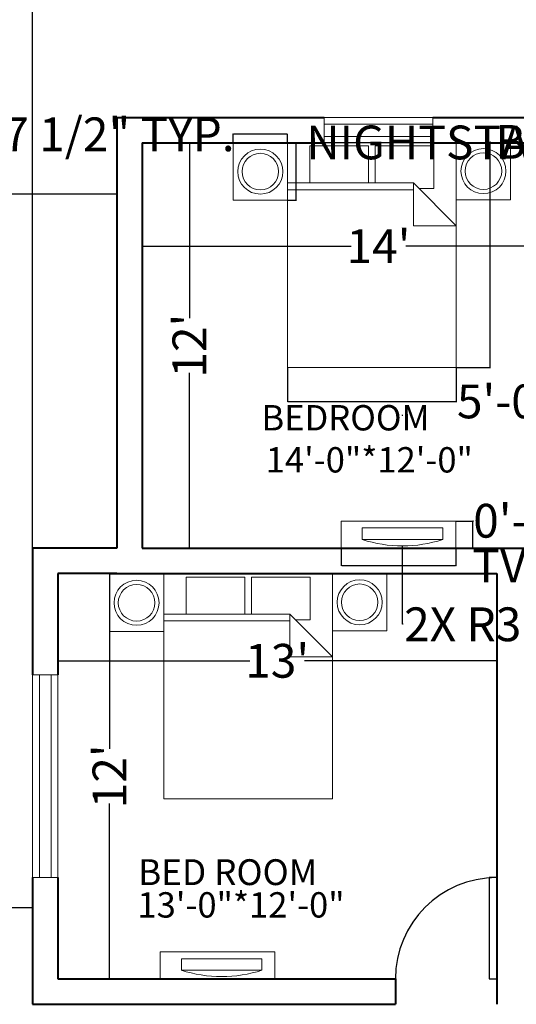
# Model space of a CAD drawing. Units: inches. Extents: x 1146 to 2917, y 889 to 2437.
# Tile 6 of 13: x 1427 to 1603, y 1867 to 2217. Entities that reach past the tile are written whole.
import ezdxf

# ---------------------------------------------------------------- set-up
doc = ezdxf.new("R2010")
doc.units = ezdxf.units.IN
doc.header["$MEASUREMENT"] = 0
for name, color, linetype, lineweight in [('A-ANNO-DIMS', 2, 'Continuous', 18), ('A-AREA-IDEN', 7, 'Continuous', 18), ('A-FURN', 9, 'Continuous', 18), ('door', 10, 'Continuous', 25), ('wall', 7, 'Continuous', 40), ('window', 5, 'Continuous', 18)]:
    doc.layers.add(name, color=color, linetype=linetype, lineweight=lineweight)
doc.styles.get("Standard").update_dxf_attribs({"font": 'arial.ttf'})
doc.dimstyles.get("Standard").update_dxf_attribs({"dimtxt": 12, "dimasz": 0.18, "dimexe": 0.18, "dimexo": 0.0625, "dimgap": 0.09, "dimtad": 0, "dimtoh": 1, "dimdec": 1, "dimzin": 0, "dimdsep": 46, "dimlunit": 4, "dimtxsty": 'Standard', "dimcen": 0.09, "dimadec": 0, "dimazin": 0, "dimtfac": 1, "dimtdec": 1, "dimtofl": 0, "dimtmove": 0, "dimatfit": 3, "dimfxl": 1, "dimtolj": 1, "dimtzin": 0, "dimarcsym": 0})

# ---------------------------------------------------------------- blocks, each defined once
blk = doc.blocks.new('*D1')
at = {"layer": 'A-ANNO-DIMS', "color": 0, "lineweight": -2, "transparency": 16777216}
for p, q in [((1314.13, 2182.33), (1314.13, 2155.05)), ((1461.13, 2182.33), (1461.13, 2155.05)), ((1314.31, 2155.23), (1367.5, 2155.23)), ((1460.95, 2155.23), (1407.77, 2155.23))]:
    blk.add_line(p, q, dxfattribs=at)
at = {"layer": 'A-ANNO-DIMS', "color": 0, "transparency": 16777216}
for points in [[(1314.31, 2155.26), (1314.31, 2155.2), (1314.13, 2155.23)], [(1460.95, 2155.26), (1460.95, 2155.2), (1461.13, 2155.23)]]:
    blk.add_solid(points, dxfattribs=at)
at = {"layer": 'Defpoints', "color": 0, "transparency": 16777216}
for p in [(1314.13, 2182.39), (1461.13, 2182.39), (1314.13, 2155.23)]:
    blk.add_point(p, dxfattribs=at)
at = {"layer": 'A-ANNO-DIMS', "color": 0, "transparency": 16777216, "insert": (1387.63, 2155.23), "char_height": 12, "attachment_point": 5}
blk.add_mtext('\\A1;12\'-3"', dxfattribs=at)
blk = doc.blocks.new('*U18')
for p, q in [((-24, 0), (-24, -6)), ((0, 0), (0, -6))]:
    blk.add_line(p, q)
blk.add_lwpolyline([(0, 0), (0, 24), (-1.75, 24), (-1.75, 0)], close=True)
blk.add_arc((0, 0), 24, 90, 180)
blk = doc.blocks.new('*D24')
at = {"layer": 'A-ANNO-DIMS', "color": 0, "lineweight": -2, "transparency": 16777216}
for p, q in [((1470.13, 2173.33), (1470.13, 2136.54)), ((1638.13, 2173.33), (1638.13, 2136.54)), ((1470.31, 2136.72), (1544.43, 2136.72)), ((1637.95, 2136.72), (1563.84, 2136.72))]:
    blk.add_line(p, q, dxfattribs=at)
at = {"layer": 'A-ANNO-DIMS', "color": 0, "transparency": 16777216}
for points in [[(1470.31, 2136.75), (1470.31, 2136.69), (1470.13, 2136.72)], [(1637.95, 2136.75), (1637.95, 2136.69), (1638.13, 2136.72)]]:
    blk.add_solid(points, dxfattribs=at)
at = {"layer": 'Defpoints', "color": 0, "transparency": 16777216}
for p in [(1470.13, 2173.39), (1638.13, 2173.39), (1638.13, 2136.72)]:
    blk.add_point(p, dxfattribs=at)
at = {"layer": 'A-ANNO-DIMS', "color": 0, "transparency": 16777216, "insert": (1554.13, 2136.72), "char_height": 12, "attachment_point": 5}
blk.add_mtext("\\A1;14'", dxfattribs=at)
blk = doc.blocks.new('*D25')
at = {"layer": 'A-ANNO-DIMS', "color": 0, "lineweight": -2, "transparency": 16777216}
for p, q in [((1470.2, 2173.39), (1487.11, 2173.39)), ((1486.93, 2173.21), (1486.93, 2111.1)), ((1486.93, 2029.57), (1486.93, 2091.68)), ((1470.2, 2029.39), (1487.11, 2029.39))]:
    blk.add_line(p, q, dxfattribs=at)
at = {"layer": 'A-ANNO-DIMS', "color": 0, "transparency": 16777216}
for points in [[(1486.9, 2173.21), (1486.96, 2173.21), (1486.93, 2173.39)], [(1486.9, 2029.57), (1486.96, 2029.57), (1486.93, 2029.39)]]:
    blk.add_solid(points, dxfattribs=at)
at = {"layer": 'Defpoints', "color": 0, "transparency": 16777216}
for p in [(1470.13, 2173.39), (1470.13, 2029.39), (1486.93, 2029.39)]:
    blk.add_point(p, dxfattribs=at)
at = {"layer": 'A-ANNO-DIMS', "color": 0, "transparency": 16777216, "insert": (1486.93, 2101.39), "char_height": 12, "attachment_point": 5, "rotation": 90}
blk.add_mtext("\\A1;12'", dxfattribs=at)
blk = doc.blocks.new('*D30')
at = {"layer": 'A-ANNO-DIMS', "color": 0, "lineweight": -2, "transparency": 16777216}
for p, q in [((1440.13, 2020.33), (1440.13, 1989.25)), ((1596.13, 2020.33), (1596.13, 1989.25)), ((1440.31, 1989.43), (1508.43, 1989.43)), ((1595.95, 1989.43), (1527.84, 1989.43))]:
    blk.add_line(p, q, dxfattribs=at)
at = {"layer": 'A-ANNO-DIMS', "color": 0, "transparency": 16777216}
for points in [[(1440.31, 1989.46), (1440.31, 1989.4), (1440.13, 1989.43)], [(1595.95, 1989.46), (1595.95, 1989.4), (1596.13, 1989.43)]]:
    blk.add_solid(points, dxfattribs=at)
at = {"layer": 'Defpoints', "color": 0, "transparency": 16777216}
for p in [(1440.13, 2020.39), (1596.13, 2020.39), (1596.13, 1989.43)]:
    blk.add_point(p, dxfattribs=at)
at = {"layer": 'A-ANNO-DIMS', "color": 0, "transparency": 16777216, "insert": (1518.13, 1989.43), "char_height": 12, "attachment_point": 5}
blk.add_mtext("\\A1;13'", dxfattribs=at)
blk = doc.blocks.new('*D31')
at = {"layer": 'A-ANNO-DIMS', "color": 0, "lineweight": -2, "transparency": 16777216}
for p, q in [((1440.2, 2020.39), (1458.71, 2020.39)), ((1458.53, 2020.21), (1458.53, 1958.1)), ((1458.53, 1876.57), (1458.53, 1938.68)), ((1440.2, 1876.39), (1458.71, 1876.39))]:
    blk.add_line(p, q, dxfattribs=at)
at = {"layer": 'A-ANNO-DIMS', "color": 0, "transparency": 16777216}
for points in [[(1458.5, 2020.21), (1458.56, 2020.21), (1458.53, 2020.39)], [(1458.5, 1876.57), (1458.56, 1876.57), (1458.53, 1876.39)]]:
    blk.add_solid(points, dxfattribs=at)
at = {"layer": 'Defpoints', "color": 0, "transparency": 16777216}
for p in [(1440.13, 2020.39), (1440.13, 1876.39), (1458.53, 1876.39)]:
    blk.add_point(p, dxfattribs=at)
at = {"layer": 'A-ANNO-DIMS', "color": 0, "transparency": 16777216, "insert": (1458.53, 1948.39), "char_height": 12, "attachment_point": 5, "rotation": 90}
blk.add_mtext("\\A1;12'", dxfattribs=at)
blk = doc.blocks.new('Bed - Queen')
for p, q in [((0, -80.00003), (0, 0)), ((0, 0), (59.99999, 0)), ((59.99999, 0), (59.99999, -80.00003)), ((7.99999, -1.2), (28.79998, -1.2)), ((7.99999, -14.4), (7.99999, -1.2)), ((28.79998, -1.2), (28.79998, -14.4)), ((31.19999, -1.2), (51.99999, -1.2)), ((31.19999, -14.4), (31.19999, -1.2)), ((51.99999, -1.2), (51.99999, -16.4)), ((0, -14.4), (44.8, -14.4)), ((44.8, -16.8), (0, -16.8)), ((59.99999, -29.6), (44.8, -14.4)), ((44.8, -14.4), (44.8, -29.6)), ((51.99999, -16.4), (46.79936, -16.4)), ((44.8, -29.6), (59.99999, -29.6)), ((59.99999, -80.00003), (0, -80.00003))]:
    blk.add_line(p, q)
blk = doc.blocks.new('*D49')
at = {"layer": 'A-ANNO-DIMS', "color": 0, "lineweight": -2, "transparency": 16777216}
for p, q in [((1314.13, 1867.45), (1314.13, 1901.79)), ((1314.31, 1901.61), (1356.59, 1901.61)), ((1430.95, 1901.61), (1388.67, 1901.61)), ((1431.13, 1867.45), (1431.13, 1901.79))]:
    blk.add_line(p, q, dxfattribs=at)
at = {"layer": 'A-ANNO-DIMS', "color": 0, "transparency": 16777216}
for points in [[(1314.31, 1901.64), (1314.31, 1901.58), (1314.13, 1901.61)], [(1430.95, 1901.64), (1430.95, 1901.58), (1431.13, 1901.61)]]:
    blk.add_solid(points, dxfattribs=at)
at = {"layer": 'Defpoints', "color": 0, "transparency": 16777216}
for p in [(1314.13, 1901.61), (1314.13, 1867.39), (1431.13, 1867.39)]:
    blk.add_point(p, dxfattribs=at)
at = {"layer": 'A-ANNO-DIMS', "color": 0, "transparency": 16777216, "insert": (1372.63, 1901.61), "char_height": 12, "attachment_point": 5}
blk.add_mtext('\\A1;9\'-9"', dxfattribs=at)
blk = doc.blocks.new('NIGHTSTAND-LAMP')
blk.add_lwpolyline([(0, 19.27), (20.36, 19.27), (20.36, 0), (0, 0)], close=True)
for radius in [8, 6.5]:
    blk.add_circle((10.18, 9.64), radius)
blk = doc.blocks.new('TV-CONSOLE-2')
for points in [[(40.71, 9.6), (40.71, 0), (0, 0), (0, 9.6)], [(36.13, 7.21), (36.13, 3.12), (7.47, 3.12), (7.47, 7.21)]]:
    blk.add_lwpolyline(points, close=True)
blk.add_arc((21.8, 47.28), 46.43, 252.0216, 287.9784)
blk = doc.blocks.new('WINDOW-PLAN-72')
for points in [[(0, 72), (9, 72), (9, 0), (0, 0)], [(2.54, 0), (6.68, 0), (6.68, 72), (2.54, 72)]]:
    blk.add_lwpolyline(points, close=True)
blk = doc.blocks.new('*D99')
at = {"layer": 'A-ANNO-DIMS', "color": 0, "lineweight": -2, "transparency": 16777216}
for p, q in [((1521.84, 2173.39), (1525.02, 2173.39)), ((1524.84, 2173.39), (1524.84, 2173.57)), ((1524.84, 2173.57), (1525.02, 2173.57)), ((1524.84, 2153.21), (1524.84, 2173.21)), ((1521.84, 2153.03), (1525.02, 2153.03))]:
    blk.add_line(p, q, dxfattribs=at)
at = {"layer": 'A-ANNO-DIMS', "color": 0, "transparency": 16777216}
for points in [[(1524.81, 2173.21), (1524.87, 2173.21), (1524.84, 2173.39)], [(1524.81, 2153.21), (1524.87, 2153.21), (1524.84, 2153.03)]]:
    blk.add_solid(points, dxfattribs=at)
at = {"layer": 'Defpoints', "color": 0, "transparency": 16777216}
for p in [(1521.78, 2173.39), (1524.84, 2173.39), (1521.78, 2153.03)]:
    blk.add_point(p, dxfattribs=at)
at = {"layer": 'A-ANNO-DIMS', "color": 0, "transparency": 16777216, "insert": (1632.18, 2173.57), "char_height": 12, "attachment_point": 5}
blk.add_mtext('\\A1;NIGHTSTAND 1\'-8 1/2" TYP.', dxfattribs=at)
blk = doc.blocks.new('*D100')
at = {"layer": 'A-ANNO-DIMS', "color": 0, "lineweight": -2, "transparency": 16777216}
for p, q in [((1502.51, 2176.45), (1502.33, 2176.45)), ((1502.51, 2173.45), (1502.51, 2176.63)), ((1521.6, 2176.45), (1502.69, 2176.45)), ((1521.78, 2173.45), (1521.78, 2176.63))]:
    blk.add_line(p, q, dxfattribs=at)
at = {"layer": 'A-ANNO-DIMS', "color": 0, "transparency": 16777216}
for points in [[(1502.69, 2176.48), (1502.69, 2176.42), (1502.51, 2176.45)], [(1521.6, 2176.48), (1521.6, 2176.42), (1521.78, 2176.45)]]:
    blk.add_solid(points, dxfattribs=at)
at = {"layer": 'Defpoints', "color": 0, "transparency": 16777216}
for p in [(1502.51, 2176.45), (1502.51, 2173.39), (1521.78, 2173.39)]:
    blk.add_point(p, dxfattribs=at)
at = {"layer": 'A-ANNO-DIMS', "color": 0, "transparency": 16777216, "insert": (1452.25, 2176.45), "char_height": 12, "attachment_point": 5}
blk.add_mtext('\\A1;1\'-7 1/2" TYP.', dxfattribs=at)
blk = doc.blocks.new('*D101')
at = {"layer": 'A-ANNO-DIMS', "color": 0, "lineweight": -2, "transparency": 16777216}
for p, q in [((1581.84, 2173.57), (1593.96, 2173.57)), ((1593.78, 2173.57), (1593.78, 2173.75)), ((1593.78, 2173.75), (1593.96, 2173.75)), ((1593.78, 2093.75), (1593.78, 2173.39)), ((1581.84, 2093.57), (1593.96, 2093.57))]:
    blk.add_line(p, q, dxfattribs=at)
at = {"layer": 'A-ANNO-DIMS', "color": 0, "transparency": 16777216}
for points in [[(1593.75, 2173.39), (1593.81, 2173.39), (1593.78, 2173.57)], [(1593.75, 2093.75), (1593.81, 2093.75), (1593.78, 2093.57)]]:
    blk.add_solid(points, dxfattribs=at)
at = {"layer": 'Defpoints', "color": 0, "transparency": 16777216}
for p in [(1581.78, 2173.57), (1593.78, 2173.57), (1581.78, 2093.57)]:
    blk.add_point(p, dxfattribs=at)
at = {"layer": 'A-ANNO-DIMS', "color": 0, "transparency": 16777216, "insert": (1649.92, 2173.75), "char_height": 12, "attachment_point": 5}
blk.add_mtext('\\A1;BED 6\'-8" TYP.', dxfattribs=at)
blk = doc.blocks.new('*D102')
at = {"layer": 'A-ANNO-DIMS', "color": 0, "lineweight": -2, "transparency": 16777216}
for p, q in [((1521.78, 2093.51), (1521.78, 2081.39)), ((1581.78, 2093.51), (1581.78, 2081.39)), ((1521.96, 2081.57), (1581.6, 2081.57)), ((1581.78, 2081.57), (1581.96, 2081.57))]:
    blk.add_line(p, q, dxfattribs=at)
at = {"layer": 'A-ANNO-DIMS', "color": 0, "transparency": 16777216}
for points in [[(1521.96, 2081.6), (1521.96, 2081.54), (1521.78, 2081.57)], [(1581.6, 2081.6), (1581.6, 2081.54), (1581.78, 2081.57)]]:
    blk.add_solid(points, dxfattribs=at)
at = {"layer": 'Defpoints', "color": 0, "transparency": 16777216}
for p in [(1521.78, 2093.57), (1581.78, 2093.57), (1581.78, 2081.57)]:
    blk.add_point(p, dxfattribs=at)
at = {"layer": 'A-ANNO-DIMS', "color": 0, "transparency": 16777216, "insert": (1618.62, 2081.57), "char_height": 12, "attachment_point": 5}
blk.add_mtext('\\A1;5\'-0" TYP.', dxfattribs=at)
blk = doc.blocks.new('*D109')
at = {"layer": 'A-ANNO-DIMS', "color": 0, "lineweight": -2, "transparency": 16777216}
for p, q in [((1540.88, 2029.33), (1540.88, 2023.11)), ((1581.59, 2029.33), (1581.59, 2023.11)), ((1541.06, 2023.29), (1581.41, 2023.29)), ((1581.59, 2023.29), (1581.77, 2023.29))]:
    blk.add_line(p, q, dxfattribs=at)
at = {"layer": 'A-ANNO-DIMS', "color": 0, "transparency": 16777216}
for points in [[(1541.06, 2023.32), (1541.06, 2023.26), (1540.88, 2023.29)], [(1581.41, 2023.32), (1581.41, 2023.26), (1581.59, 2023.29)]]:
    blk.add_solid(points, dxfattribs=at)
at = {"layer": 'Defpoints', "color": 0, "transparency": 16777216}
for p in [(1540.88, 2029.39), (1581.59, 2029.39), (1581.59, 2023.29)]:
    blk.add_point(p, dxfattribs=at)
at = {"layer": 'A-ANNO-DIMS', "color": 0, "transparency": 16777216, "insert": (1688.92, 2023.29), "char_height": 12, "attachment_point": 5}
blk.add_mtext('\\A1;TV CONSOLE 3\'-4 1/2" TYP.', dxfattribs=at)
blk = doc.blocks.new('*D110')
at = {"layer": 'A-ANNO-DIMS', "color": 0, "lineweight": -2, "transparency": 16777216}
for p, q in [((1581.65, 2038.99), (1587.87, 2038.99)), ((1587.69, 2038.99), (1587.69, 2039.17)), ((1587.69, 2039.17), (1587.87, 2039.17)), ((1587.69, 2029.57), (1587.69, 2038.81)), ((1581.65, 2029.39), (1587.87, 2029.39))]:
    blk.add_line(p, q, dxfattribs=at)
at = {"layer": 'A-ANNO-DIMS', "color": 0, "transparency": 16777216}
for points in [[(1587.66, 2038.81), (1587.72, 2038.81), (1587.69, 2038.99)], [(1587.66, 2029.57), (1587.72, 2029.57), (1587.69, 2029.39)]]:
    blk.add_solid(points, dxfattribs=at)
at = {"layer": 'Defpoints', "color": 0, "transparency": 16777216}
for p in [(1581.59, 2038.99), (1587.69, 2038.99), (1581.59, 2029.39)]:
    blk.add_point(p, dxfattribs=at)
at = {"layer": 'A-ANNO-DIMS', "color": 0, "transparency": 16777216, "insert": (1638.52, 2039.17), "char_height": 12, "attachment_point": 5}
blk.add_mtext('\\A1;0\'-9 1/2" TYP.', dxfattribs=at)
blk = doc.blocks.new('*D168')
at = {"layer": 'A-ANNO-DIMS', "color": 0, "lineweight": -2, "transparency": 16777216}
for p, q in [((1431.13, 2029.45), (1431.13, 2426.57)), ((1431.31, 2426.39), (1674.19, 2426.39)), ((1958.95, 2426.39), (1716.08, 2426.39)), ((1959.13, 2029.45), (1959.13, 2426.57))]:
    blk.add_line(p, q, dxfattribs=at)
at = {"layer": 'A-ANNO-DIMS', "color": 0, "transparency": 16777216}
for points in [[(1431.31, 2426.42), (1431.31, 2426.36), (1431.13, 2426.39)], [(1958.95, 2426.42), (1958.95, 2426.36), (1959.13, 2426.39)]]:
    blk.add_solid(points, dxfattribs=at)
at = {"layer": 'Defpoints', "color": 0, "transparency": 16777216}
for p in [(1959.13, 2426.39), (1431.13, 2029.39), (1959.13, 2029.39)]:
    blk.add_point(p, dxfattribs=at)
at = {"layer": 'A-ANNO-DIMS', "color": 0, "transparency": 16777216, "insert": (1695.13, 2426.39), "char_height": 12, "attachment_point": 5}
blk.add_mtext('\\A1;44\'-0"', dxfattribs=at)
blk = doc.blocks.new('*D178')
at = {"layer": 'A-ANNO-DIMS', "color": 0, "lineweight": -2, "transparency": 16777216}
for p, q in [((1562.58, 2076.67), (1562.76, 2076.67)), ((1562.67, 2076.58), (1562.67, 2076.76)), ((1562.67, 2002.39), (1562.67, 2030.07)), ((1562.85, 2002.39), (1562.67, 2002.39))]:
    blk.add_line(p, q, dxfattribs=at)
at = {"layer": 'A-ANNO-DIMS', "color": 0, "transparency": 16777216}
blk.add_solid([(1562.7, 2030.07), (1562.64, 2030.07), (1562.67, 2030.25)], dxfattribs=at)
at = {"layer": 'Defpoints', "color": 0, "transparency": 16777216}
for p in [(1562.67, 2076.67), (1562.67, 2030.25)]:
    blk.add_point(p, dxfattribs=at)
at = {"layer": 'A-ANNO-DIMS', "color": 0, "transparency": 16777216, "insert": (1616.27, 2002.39), "char_height": 12, "attachment_point": 5}
blk.add_mtext('\\A1;2X R3\'-10 1/2"', dxfattribs=at)

msp = doc.modelspace()

# ---------------------------------------------------------------- linework, layer by layer
at = {"layer": 'wall'}
for p, q in [((1461.13, 2182.39), (1534.88, 2182.39)), ((1461.13, 2182.39), (1461.13, 2029.39)), ((1573.38, 2182.39), (1680.13, 2182.39)), ((1470.13, 2173.39), (1470.13, 2029.39)), ((1470.13, 2173.39), (1534.88, 2173.39)), ((1573.38, 2173.39), (1638.13, 2173.39)), ((1461.13, 2029.39), (1431.13, 2029.39)), ((1431.13, 2029.39), (1431.13, 1984.39)), ((1470.13, 2029.39), (1662.13, 2029.39)), ((1461.13, 2020.39), (1440.13, 2020.39)), ((1440.13, 2020.39), (1440.13, 1984.39)), ((1461.13, 2020.39), (1596.13, 2020.39)), ((1596.13, 2020.39), (1596.13, 1867.39)), ((1431.13, 1912.39), (1431.13, 1867.39)), ((1440.13, 1912.39), (1440.13, 1876.39)), ((1440.13, 1876.39), (1560.13, 1876.39)), ((1560.13, 1876.39), (1560.13, 1867.39)), ((1431.13, 1867.39), (1560.13, 1867.39))]:
    msp.add_line(p, q, dxfattribs=at)
at = {"layer": 'window'}
msp.add_line((1573.38, 2182.39), (1534.88, 2182.39), dxfattribs=at)
msp.add_lwpolyline([(1573.38, 2182.39), (1573.38, 2173.39), (1534.88, 2173.39), (1534.88, 2182.39)], dxfattribs=at)
msp.add_lwpolyline([(1534.88, 2180.1), (1573.38, 2180.1), (1573.38, 2175.69), (1534.88, 2175.69)], close=True, dxfattribs=at)

# ---------------------------------------------------------------- block references
at = {"layer": 'A-FURN'}
for p, rotation in [((1521.78, 2153.03), 89.99999999999811), ((1601.05, 2153.21), 89.99999999999883), ((1477.81, 1999.85), 89.99999999999756), ((1557.08, 2000.03), 90.00000000000003)]:
    msp.add_blockref('NIGHTSTAND-LAMP', p, dxfattribs=dict(at, rotation=rotation))
for name, p in [('Bed - Queen', (1521.78, 2173.57)), ('TV-CONSOLE-2', (1540.88, 2029.39)), ('Bed - Queen', (1477.81, 2020.39)), ('TV-CONSOLE-2', (1476.6, 1876.39))]:
    msp.add_blockref(name, p, dxfattribs=at)
at = {"layer": 'door', "xscale": 1.500000000000009, "yscale": 1.500000000000009, "zscale": 1.500000000000009}
msp.add_blockref('*U18', (1596.13, 1876.39), dxfattribs=at)
at = {"layer": 'window'}
msp.add_blockref('WINDOW-PLAN-72', (1431.13, 1912.39), dxfattribs=at)

# ---------------------------------------------------------------- texts
at = {"layer": 'A-AREA-IDEN', "attachment_point": 1}
for s, width, gutter_width, insert, char_height in [('BEDROOM', 90.7924, 1, (1512.55, 2080.26), 9), ('14\'-0"*12\'-0"', 76.36, 1, (1514.07, 2065.32), 9), ('BED ROOM', 4038.7012, 45.86, (1468.71, 1918.92), 9.172), ('13\'-0"*12\'-0"', 70.5587, 1, (1468.48, 1907.21), 9)]:
    msp.add_mtext_dynamic_manual_height_columns(s, width=width, gutter_width=gutter_width, heights=[0], dxfattribs=dict(at, insert=insert, char_height=char_height))

# ---------------------------------------------------------------- dimensions: what is measured, and where the dimension line sits
at = {"layer": 'A-ANNO-DIMS'}
dim = msp.add_linear_dim(base=(1959.13, 2426.39), p1=(1431.13, 2029.39), p2=(1959.13, 2029.39), dimstyle='Standard', override={"dimdec": 1, "dimlfac": 1, "dimrnd": 0, "dimzin": 1, "dimdsep": 46, "dimlunit": 4, "dimfrac": 2}, dxfattribs=at)
dim.commit()
dim.dimension.update_dxf_attribs({"geometry": '*D168', "text_midpoint": (1695.13, 2426.39)})
for base, p1, p2, angle, text, picture, middle in [((1524.84, 2173.39), (1521.78, 2153.03), (1521.78, 2173.39), 90, 'NIGHTSTAND <> TYP.', '*D99', (1632.18, 2173.57)), ((1502.51, 2176.45), (1521.78, 2173.39), (1502.51, 2173.39), 180, '<> TYP.', '*D100', (1452.25, 2176.45)), ((1593.78, 2173.57), (1581.78, 2093.57), (1581.78, 2173.57), 90, 'BED <> TYP.', '*D101', (1649.92, 2173.75)), ((1587.69, 2038.99), (1581.59, 2029.39), (1581.59, 2038.99), 90, '<> TYP.', '*D110', (1638.52, 2039.17))]:
    dim = msp.add_linear_dim(base=base, p1=p1, p2=p2, angle=angle, text=text, dimstyle='Standard', override={"dimdec": 1, "dimlfac": 1, "dimrnd": 0, "dimzin": 1, "dimdsep": 46, "dimlunit": 4, "dimfrac": 2}, dxfattribs=at)
    dim.commit()
    dim.dimension.update_dxf_attribs({"geometry": picture, "text_midpoint": middle})
for p1, p2, distance, picture, middle in [((1461.13, 2182.39), (1314.13, 2182.39), 27.16, '*D1', (1387.63, 2155.23)), ((1470.13, 2173.39), (1638.13, 2173.39), -36.67, '*D24', (1554.13, 2136.72)), ((1470.13, 2173.39), (1470.13, 2029.39), 16.79, '*D25', (1486.93, 2101.39)), ((1440.13, 2020.39), (1596.13, 2020.39), -30.96, '*D30', (1518.13, 1989.43)), ((1440.13, 2020.39), (1440.13, 1876.39), 18.4, '*D31', (1458.53, 1948.39)), ((1431.13, 1867.39), (1314.13, 1867.39), -34.21, '*D49', (1372.63, 1901.61))]:
    dim = msp.add_aligned_dim(p1=p1, p2=p2, distance=distance, dimstyle='Standard', override={"dimclrd": 0, "dimclre": 0, "dimclrt": 0}, dxfattribs=at)
    dim.commit()
    dim.dimension.update_dxf_attribs({"geometry": picture, "text_midpoint": middle})
for base, p1, p2, text, picture, middle in [((1581.78, 2081.57), (1521.78, 2093.57), (1581.78, 2093.57), '<> TYP.', '*D102', (1618.62, 2081.57)), ((1581.59, 2023.29), (1540.88, 2029.39), (1581.59, 2029.39), 'TV CONSOLE <> TYP.', '*D109', (1688.92, 2023.29))]:
    dim = msp.add_linear_dim(base=base, p1=p1, p2=p2, text=text, dimstyle='Standard', override={"dimdec": 1, "dimlfac": 1, "dimrnd": 0, "dimzin": 1, "dimdsep": 46, "dimlunit": 4, "dimfrac": 2}, dxfattribs=at)
    dim.commit()
    dim.dimension.update_dxf_attribs({"geometry": picture, "text_midpoint": middle})
dim = msp.add_radius_dim(center=(1562.67, 2076.67), mpoint=(1562.67, 2030.25), text='2X <>', dimstyle='Standard', override={"dimdec": 1, "dimlfac": 1, "dimrnd": 0, "dimzin": 1, "dimdsep": 46, "dimlunit": 4, "dimfrac": 2}, dxfattribs=at)
dim.commit()
dim.dimension.update_dxf_attribs({"geometry": '*D178', "text_midpoint": (1616.27, 2002.39), "dimtype": 164})

doc.saveas('drawing.dxf')
